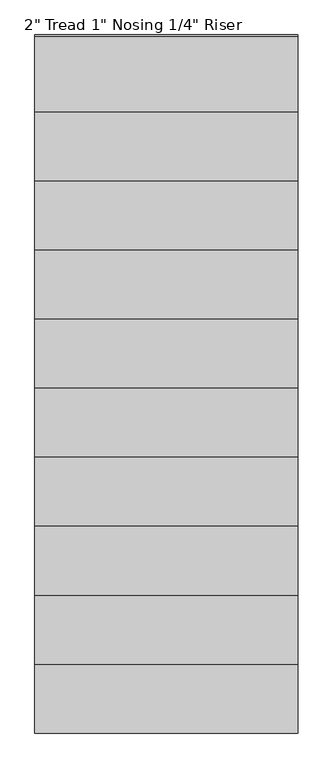
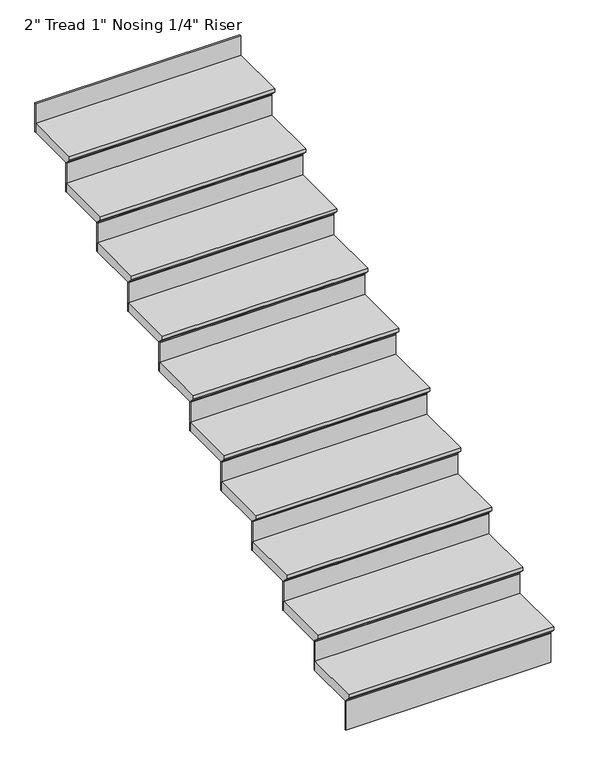
"""IFC4 building model written with IfcOpenShell, lengths in millimetres: stair flight geometry."""

from ifc_helpers import new_model, si_unit, frame, origin, place, context, project, spatial, polyline, outline, extrude, source, transform, mapped, element, save


def stair_flight_ccf2217f(model_context):
    return source(origin(), model_context, "Body", "SweptSolid", [
        extrude(outline(polyline([(4095.086641, 1911.9272727), (4399.886641, 1911.9272727), (4399.886641, 1861.1272727), (4120.486641, 1861.1272727), (4120.486641, 1867.4772727), (4095.086641, 1892.8772727), (4095.086641, 1911.9272727)])), frame((-8032.1581554, 0.0, 0.0), z_axis=(1.0, 0.0, 0.0), x_axis=(0.0, 1.0, 0.0)), (0.0, 0.0, 1.0), 1066.8),
        extrude(outline(polyline([(-6965.3581554, 4126.836641), (-6965.3581554, 4120.486641), (-8032.1581554, 4120.486641), (-8032.1581554, 4126.836641), (-6965.3581554, 4126.836641)])), frame((0.0, 0.0, 1701.8), z_axis=(0.0, 0.0, 1.0), x_axis=(1.0, 0.0, 0.0)), (0.0, 0.0, 1.0), 159.3272727),
        extrude(outline(polyline([(-6965.3581554, 4406.236641), (-6965.3581554, 4399.886641), (-8032.1581554, 4399.886641), (-8032.1581554, 4406.236641), (-6965.3581554, 4406.236641)])), frame((0.0, 0.0, 1861.1272727), z_axis=(0.0, 0.0, 1.0), x_axis=(1.0, 0.0, 0.0)), (0.0, 0.0, 1.0), 159.3272727),
        extrude(outline(polyline([(4374.486641, 2071.2545455), (4679.286641, 2071.2545455), (4679.286641, 2020.4545455), (4399.886641, 2020.4545455), (4399.886641, 2026.8045455), (4374.486641, 2052.2045455), (4374.486641, 2071.2545455)])), frame((-8032.1581554, 0.0, 0.0), z_axis=(1.0, 0.0, 0.0), x_axis=(0.0, 1.0, 0.0)), (0.0, 0.0, 1.0), 1066.8),
        extrude(outline(polyline([(-6965.3581554, 4685.636641), (-6965.3581554, 4679.286641), (-8032.1581554, 4679.286641), (-8032.1581554, 4685.636641), (-6965.3581554, 4685.636641)])), frame((0.0, 0.0, 2020.4545455), z_axis=(0.0, 0.0, 1.0), x_axis=(1.0, 0.0, 0.0)), (0.0, 0.0, 1.0), 159.3272727),
        extrude(outline(polyline([(4653.886641, 2230.5818182), (4958.686641, 2230.5818182), (4958.686641, 2179.7818182), (4679.286641, 2179.7818182), (4679.286641, 2186.1318182), (4653.886641, 2211.5318182), (4653.886641, 2230.5818182)])), frame((-8032.1581554, 0.0, 0.0), z_axis=(1.0, 0.0, 0.0), x_axis=(0.0, 1.0, 0.0)), (0.0, 0.0, 1.0), 1066.8),
        extrude(outline(polyline([(-6965.3581554, 4965.036641), (-6965.3581554, 4958.686641), (-8032.1581554, 4958.686641), (-8032.1581554, 4965.036641), (-6965.3581554, 4965.036641)])), frame((0.0, 0.0, 2179.7818182), z_axis=(0.0, 0.0, 1.0), x_axis=(1.0, 0.0, 0.0)), (0.0, 0.0, 1.0), 159.3272727),
        extrude(outline(polyline([(4933.286641, 2389.9090909), (5238.086641, 2389.9090909), (5238.086641, 2339.1090909), (4958.686641, 2339.1090909), (4958.686641, 2345.4590909), (4933.286641, 2370.8590909), (4933.286641, 2389.9090909)])), frame((-8032.1581554, 0.0, 0.0), z_axis=(1.0, 0.0, 0.0), x_axis=(0.0, 1.0, 0.0)), (0.0, 0.0, 1.0), 1066.8),
        extrude(outline(polyline([(-6965.3581554, 5244.436641), (-6965.3581554, 5238.086641), (-8032.1581554, 5238.086641), (-8032.1581554, 5244.436641), (-6965.3581554, 5244.436641)])), frame((0.0, 0.0, 2339.1090909), z_axis=(0.0, 0.0, 1.0), x_axis=(1.0, 0.0, 0.0)), (0.0, 0.0, 1.0), 159.3272727),
        extrude(outline(polyline([(5212.686641, 2549.2363636), (5517.486641, 2549.2363636), (5517.486641, 2498.4363636), (5238.086641, 2498.4363636), (5238.086641, 2504.7863636), (5212.686641, 2530.1863636), (5212.686641, 2549.2363636)])), frame((-8032.1581554, 0.0, 0.0), z_axis=(1.0, 0.0, 0.0), x_axis=(0.0, 1.0, 0.0)), (0.0, 0.0, 1.0), 1066.8),
        extrude(outline(polyline([(-6965.3581554, 5523.836641), (-6965.3581554, 5517.486641), (-8032.1581554, 5517.486641), (-8032.1581554, 5523.836641), (-6965.3581554, 5523.836641)])), frame((0.0, 0.0, 2498.4363636), z_axis=(0.0, 0.0, 1.0), x_axis=(1.0, 0.0, 0.0)), (0.0, 0.0, 1.0), 159.3272727),
        extrude(outline(polyline([(5492.086641, 2708.5636364), (5796.886641, 2708.5636364), (5796.886641, 2657.7636364), (5517.486641, 2657.7636364), (5517.486641, 2664.1136364), (5492.086641, 2689.5136364), (5492.086641, 2708.5636364)])), frame((-8032.1581554, 0.0, 0.0), z_axis=(1.0, 0.0, 0.0), x_axis=(0.0, 1.0, 0.0)), (0.0, 0.0, 1.0), 1066.8),
        extrude(outline(polyline([(-6965.3581554, 5803.236641), (-6965.3581554, 5796.886641), (-8032.1581554, 5796.886641), (-8032.1581554, 5803.236641), (-6965.3581554, 5803.236641)])), frame((0.0, 0.0, 2657.7636364), z_axis=(0.0, 0.0, 1.0), x_axis=(1.0, 0.0, 0.0)), (0.0, 0.0, 1.0), 159.3272727),
        extrude(outline(polyline([(5771.486641, 2867.8909091), (6076.286641, 2867.8909091), (6076.286641, 2817.0909091), (5796.886641, 2817.0909091), (5796.886641, 2823.4409091), (5771.486641, 2848.8409091), (5771.486641, 2867.8909091)])), frame((-8032.1581554, 0.0, 0.0), z_axis=(1.0, 0.0, 0.0), x_axis=(0.0, 1.0, 0.0)), (0.0, 0.0, 1.0), 1066.8),
        extrude(outline(polyline([(-6965.3581554, 6082.636641), (-6965.3581554, 6076.286641), (-8032.1581554, 6076.286641), (-8032.1581554, 6082.636641), (-6965.3581554, 6082.636641)])), frame((0.0, 0.0, 2817.0909091), z_axis=(0.0, 0.0, 1.0), x_axis=(1.0, 0.0, 0.0)), (0.0, 0.0, 1.0), 159.3272727),
        extrude(outline(polyline([(6050.886641, 3027.2181818), (6355.686641, 3027.2181818), (6355.686641, 2976.4181818), (6076.286641, 2976.4181818), (6076.286641, 2982.7681818), (6050.886641, 3008.1681818), (6050.886641, 3027.2181818)])), frame((-8032.1581554, 0.0, 0.0), z_axis=(1.0, 0.0, 0.0), x_axis=(0.0, 1.0, 0.0)), (0.0, 0.0, 1.0), 1066.8),
        extrude(outline(polyline([(-6965.3581554, 6362.036641), (-6965.3581554, 6355.686641), (-8032.1581554, 6355.686641), (-8032.1581554, 6362.036641), (-6965.3581554, 6362.036641)])), frame((0.0, 0.0, 2976.4181818), z_axis=(0.0, 0.0, 1.0), x_axis=(1.0, 0.0, 0.0)), (0.0, 0.0, 1.0), 159.3272727),
        extrude(outline(polyline([(6330.286641, 3186.5454545), (6635.086641, 3186.5454545), (6635.086641, 3135.7454545), (6355.686641, 3135.7454545), (6355.686641, 3142.0954545), (6330.286641, 3167.4954545), (6330.286641, 3186.5454545)])), frame((-8032.1581554, 0.0, 0.0), z_axis=(1.0, 0.0, 0.0), x_axis=(0.0, 1.0, 0.0)), (0.0, 0.0, 1.0), 1066.8),
        extrude(outline(polyline([(-6965.3581554, 6641.436641), (-6965.3581554, 6635.086641), (-8032.1581554, 6635.086641), (-8032.1581554, 6641.436641), (-6965.3581554, 6641.436641)])), frame((0.0, 0.0, 3135.7454545), z_axis=(0.0, 0.0, 1.0), x_axis=(1.0, 0.0, 0.0)), (0.0, 0.0, 1.0), 159.3272727),
        extrude(outline(polyline([(-6965.3581554, 6920.836641), (-6965.3581554, 6914.486641), (-8032.1581554, 6914.486641), (-8032.1581554, 6920.836641), (-6965.3581554, 6920.836641)])), frame((0.0, 0.0, 3295.0727273), z_axis=(0.0, 0.0, 1.0), x_axis=(1.0, 0.0, 0.0)), (0.0, 0.0, 1.0), 159.3272727),
        extrude(outline(polyline([(6609.686641, 3345.8727273), (6914.486641, 3345.8727273), (6914.486641, 3295.0727273), (6635.086641, 3295.0727273), (6635.086641, 3301.4227273), (6609.686641, 3326.8227273), (6609.686641, 3345.8727273)])), frame((-8032.1581554, 0.0, 0.0), z_axis=(1.0, 0.0, 0.0), x_axis=(0.0, 1.0, 0.0)), (0.0, 0.0, 1.0), 1066.8),
    ])


if __name__ == "__main__":
    model = new_model("IFC4")
    model_context = context("Model", 3, world=origin())
    ifc_project = project(units=[si_unit("LENGTHUNIT", "METRE", prefix="MILLI")], contexts=[model_context])
    site = spatial("IfcSite", under=ifc_project)
    building = spatial("IfcBuilding", under=site)
    placement = place(None, origin())
    stair_flight_shape = stair_flight_ccf2217f(model_context)
    element("IfcStairFlight", 1, ObjectType="2\" Tread 1\" Nosing 1/4\" Riser", at=placement, inside=building, context=model_context, shape_type="MappedRepresentation", body=[
        mapped(stair_flight_shape, transform((0.0, 0.0, 0.0), x_axis=(1.0, 0.0, 0.0), y_axis=(0.0, 1.0, 0.0), z_axis=(0.0, 0.0, 1.0))),
    ])
    save(model, "model.ifc")
